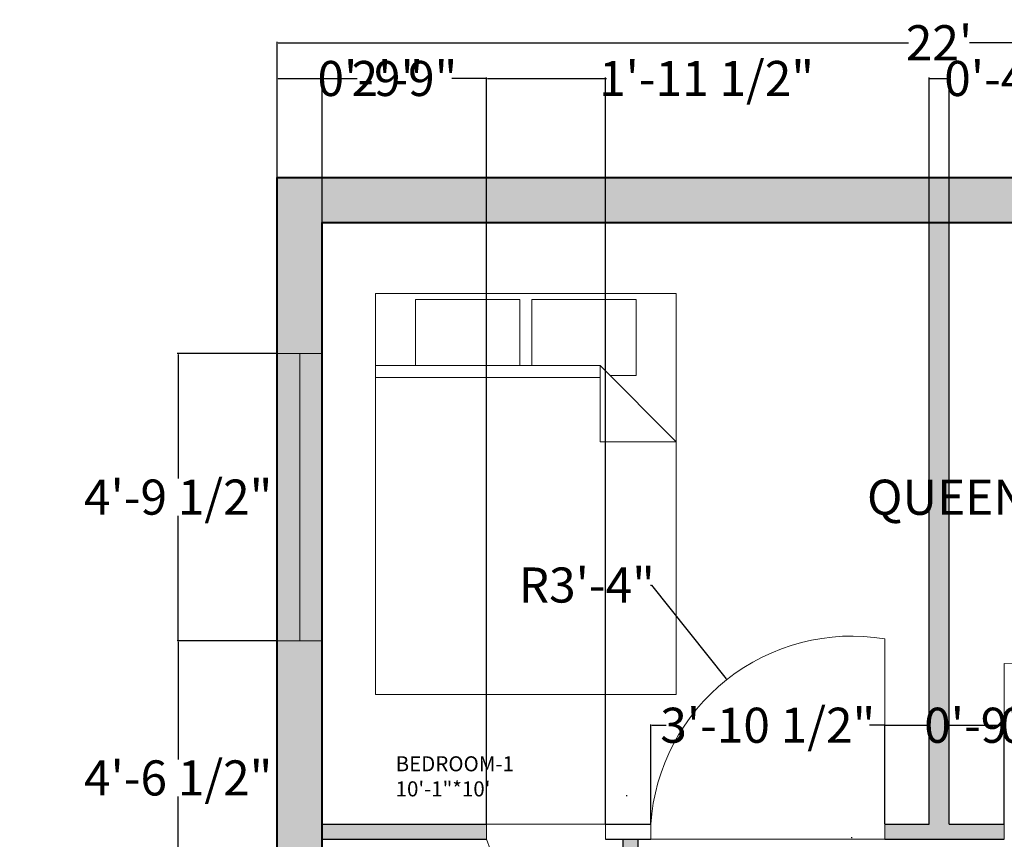
# Model space of a CAD drawing. Units: inches. Extents: x 4466 to 4826, y 3691 to 4152.
# Tile 3 of 4: x 4466 to 4663, y 3988 to 4152. Entities that reach past the tile are written whole.
import ezdxf

# ---------------------------------------------------------------- set-up
doc = ezdxf.new("R2010")
doc.units = ezdxf.units.IN
doc.header["$MEASUREMENT"] = 0
for name, color, linetype, lineweight in [('A-ANNO-DIMS', 2, 'Continuous', 13), ('A-DOOR', 3, 'Continuous', 18), ('A-FLOR-FIXT', 8, 'Continuous', 18), ('A-GLAZ', 4, 'Continuous', 13), ('A-GLAZ-PATT', 9, 'Continuous', 13), ('A-TEXT-ROOM', 7, 'Continuous', 18), ('A-WALL-EXTR', 7, 'Continuous', 40), ('A-WALL-INTR', 7, 'Continuous', 25), ('A-WALL-PATT', 251, 'Continuous', 13)]:
    doc.layers.add(name, color=color, linetype=linetype, lineweight=lineweight)
doc.styles.get("Standard").update_dxf_attribs({"font": 'arial.ttf'})
doc.dimstyles.get("Standard").update_dxf_attribs({"dimtxt": 7, "dimasz": 0.18, "dimexe": 0.18, "dimexo": 0.0625, "dimgap": 0.09, "dimtad": 0, "dimtih": 1, "dimtoh": 1, "dimdec": 0, "dimzin": 0, "dimdsep": 46, "dimlunit": 3, "dimtxsty": 'Standard', "dimcen": 0.09, "dimadec": 0, "dimazin": 0, "dimtfac": 1, "dimtdec": 0, "dimtofl": 0, "dimtmove": 0, "dimatfit": 3, "dimfxl": 1, "dimtolj": 1, "dimtzin": 0, "dimarcsym": 0})

# ---------------------------------------------------------------- blocks, each defined once
blk = doc.blocks.new('Bed - Queen')
for p, q in [((0, -80.00003), (0, 0)), ((0, 0), (59.99999, 0)), ((59.99999, 0), (59.99999, -80.00003)), ((7.99999, -1.2), (28.79998, -1.2)), ((7.99999, -14.4), (7.99999, -1.2)), ((28.79998, -1.2), (28.79998, -14.4)), ((31.19999, -1.2), (51.99999, -1.2)), ((31.19999, -14.4), (31.19999, -1.2)), ((51.99999, -1.2), (51.99999, -16.4)), ((0, -14.4), (44.8, -14.4)), ((59.99999, -29.6), (44.8, -14.4)), ((44.8, -14.4), (44.8, -29.6)), ((44.8, -16.8), (0, -16.8)), ((51.99999, -16.4), (46.79936, -16.4)), ((44.8, -29.6), (59.99999, -29.6)), ((59.99999, -80.00003), (0, -80.00003))]:
    blk.add_line(p, q)
blk = doc.blocks.new('*D7')
at = {"layer": 'A-ANNO-DIMS', "color": 0, "lineweight": -2, "transparency": 16777216}
for p, q in [((4517.73, 4120.34), (4517.73, 4147.34)), ((4517.91, 4147.16), (4643.64, 4147.16)), ((4781.55, 4147.16), (4655.82, 4147.16)), ((4781.73, 4120.34), (4781.73, 4147.34))]:
    blk.add_line(p, q, dxfattribs=at)
at = {"layer": 'A-ANNO-DIMS', "color": 0, "transparency": 16777216}
for points in [[(4517.91, 4147.19), (4517.91, 4147.13), (4517.73, 4147.16)], [(4781.55, 4147.19), (4781.55, 4147.13), (4781.73, 4147.16)]]:
    blk.add_solid(points, dxfattribs=at)
at = {"layer": 'Defpoints', "color": 0, "transparency": 16777216}
for p in [(4781.73, 4147.16), (4517.73, 4120.28), (4781.73, 4120.28)]:
    blk.add_point(p, dxfattribs=at)
at = {"layer": 'A-ANNO-DIMS', "color": 0, "transparency": 16777216, "insert": (4649.73, 4147.16), "char_height": 7, "attachment_point": 5}
blk.add_mtext("\\A1;22'", dxfattribs=at)
blk = doc.blocks.new('*D8')
at = {"layer": 'A-ANNO-DIMS', "color": 0, "lineweight": -2, "transparency": 16777216}
for p, q in [((4696.1, 4096.51), (4683.98, 4096.51)), ((4684.16, 4096.33), (4684.16, 4060.43)), ((4684.16, 4016.69), (4684.16, 4052.59)), ((4696.1, 4016.51), (4683.98, 4016.51))]:
    blk.add_line(p, q, dxfattribs=at)
at = {"layer": 'A-ANNO-DIMS', "color": 0, "transparency": 16777216}
for points in [[(4684.13, 4096.33), (4684.19, 4096.33), (4684.16, 4096.51)], [(4684.13, 4016.69), (4684.19, 4016.69), (4684.16, 4016.51)]]:
    blk.add_solid(points, dxfattribs=at)
at = {"layer": 'Defpoints', "color": 0, "transparency": 16777216}
for p in [(4684.16, 4096.51), (4696.16, 4096.51), (4696.16, 4016.51)]:
    blk.add_point(p, dxfattribs=at)
at = {"layer": 'A-ANNO-DIMS', "color": 0, "transparency": 16777216, "insert": (4684.16, 4056.51), "char_height": 7, "attachment_point": 5}
blk.add_mtext('\\A1;QUEEN BED 6\'-8" TYP.', dxfattribs=at)
blk = doc.blocks.new('*D10')
at = {"layer": 'A-ANNO-DIMS', "color": 0, "lineweight": -2, "transparency": 16777216}
for p, q in [((4527.05, 3975.44), (4526.87, 3975.44)), ((4527.05, 3970.54), (4527.05, 3975.62)), ((4559.92, 3975.44), (4527.23, 3975.44)), ((4560.1, 3970.54), (4560.1, 3975.62))]:
    blk.add_line(p, q, dxfattribs=at)
at = {"layer": 'A-ANNO-DIMS', "color": 0, "transparency": 16777216}
for points in [[(4527.23, 3975.47), (4527.23, 3975.41), (4527.05, 3975.44)], [(4559.92, 3975.47), (4559.92, 3975.41), (4560.1, 3975.44)]]:
    blk.add_solid(points, dxfattribs=at)
at = {"layer": 'Defpoints', "color": 0, "transparency": 16777216}
for p in [(4527.05, 3975.44), (4527.05, 3970.48), (4560.1, 3970.48)]:
    blk.add_point(p, dxfattribs=at)
at = {"layer": 'A-ANNO-DIMS', "color": 0, "transparency": 16777216, "insert": (4495.8, 3975.44), "char_height": 7, "attachment_point": 5}
blk.add_mtext('\\A1;WC 2\'-9" TYP.', dxfattribs=at)
blk = doc.blocks.new('*D26')
at = {"layer": 'A-ANNO-DIMS', "color": 0, "lineweight": -2, "transparency": 16777216}
for p, q in [((4517.67, 4027.88), (4497.8, 4027.88)), ((4497.98, 4027.7), (4497.98, 4004.23)), ((4497.98, 3973.33), (4497.98, 3996.81)), ((4517.67, 3973.15), (4497.8, 3973.15))]:
    blk.add_line(p, q, dxfattribs=at)
at = {"layer": 'A-ANNO-DIMS', "color": 0, "transparency": 16777216}
for points in [[(4497.95, 4027.7), (4498.01, 4027.7), (4497.98, 4027.88)], [(4497.95, 3973.33), (4498.01, 3973.33), (4497.98, 3973.15)]]:
    blk.add_solid(points, dxfattribs=at)
at = {"layer": 'Defpoints', "color": 0, "transparency": 16777216}
for p in [(4497.98, 4027.88), (4517.73, 4027.88), (4517.73, 3973.15)]:
    blk.add_point(p, dxfattribs=at)
at = {"layer": 'A-ANNO-DIMS', "color": 0, "transparency": 16777216, "insert": (4497.98, 4000.52), "char_height": 7, "attachment_point": 5}
blk.add_mtext('\\A1;4\'-6 1/2"', dxfattribs=at)
blk = doc.blocks.new('*D27')
at = {"layer": 'A-ANNO-DIMS', "color": 0, "lineweight": -2, "transparency": 16777216}
for p, q in [((4517.67, 4085.19), (4497.8, 4085.19)), ((4497.98, 4085.01), (4497.98, 4060.24)), ((4497.98, 4028.06), (4497.98, 4052.82)), ((4517.67, 4027.88), (4497.8, 4027.88))]:
    blk.add_line(p, q, dxfattribs=at)
at = {"layer": 'A-ANNO-DIMS', "color": 0, "transparency": 16777216}
for points in [[(4497.95, 4085.01), (4498.01, 4085.01), (4497.98, 4085.19)], [(4497.95, 4028.06), (4498.01, 4028.06), (4497.98, 4027.88)]]:
    blk.add_solid(points, dxfattribs=at)
at = {"layer": 'Defpoints', "color": 0, "transparency": 16777216}
for p in [(4497.98, 4085.19), (4517.73, 4085.19), (4517.73, 4027.88)]:
    blk.add_point(p, dxfattribs=at)
at = {"layer": 'A-ANNO-DIMS', "color": 0, "transparency": 16777216, "insert": (4497.98, 4056.53), "char_height": 7, "attachment_point": 5}
blk.add_mtext('\\A1;4\'-9 1/2"', dxfattribs=at)
blk = doc.blocks.new('*D44')
at = {"layer": 'A-ANNO-DIMS', "color": 0, "lineweight": -2, "transparency": 16777216}
for p, q in [((4559.49, 3991.34), (4559.49, 4140.21)), ((4559.67, 4140.03), (4583.06, 4140.03)), ((4583.24, 3991.34), (4583.24, 4140.21)), ((4583.24, 4140.03), (4583.42, 4140.03))]:
    blk.add_line(p, q, dxfattribs=at)
at = {"layer": 'A-ANNO-DIMS', "color": 0, "transparency": 16777216}
for points in [[(4559.67, 4140.06), (4559.67, 4140), (4559.49, 4140.03)], [(4583.06, 4140.06), (4583.06, 4140), (4583.24, 4140.03)]]:
    blk.add_solid(points, dxfattribs=at)
at = {"layer": 'Defpoints', "color": 0, "transparency": 16777216}
for p in [(4583.24, 4140.03), (4559.49, 3991.28), (4583.24, 3991.28)]:
    blk.add_point(p, dxfattribs=at)
at = {"layer": 'A-ANNO-DIMS', "color": 0, "transparency": 16777216, "insert": (4603.36, 4140.03), "char_height": 7, "attachment_point": 5}
blk.add_mtext('\\A1;1\'-11 1/2"', dxfattribs=at)
blk = doc.blocks.new('*D45')
at = {"layer": 'A-ANNO-DIMS', "color": 0, "lineweight": -2, "transparency": 16777216}
for p, q in [((4526.73, 3991.34), (4526.73, 4140.21)), ((4526.91, 4140.03), (4533.66, 4140.03)), ((4559.31, 4140.03), (4552.57, 4140.03)), ((4559.49, 3991.34), (4559.49, 4140.21))]:
    blk.add_line(p, q, dxfattribs=at)
at = {"layer": 'A-ANNO-DIMS', "color": 0, "transparency": 16777216}
for points in [[(4526.91, 4140.06), (4526.91, 4140), (4526.73, 4140.03)], [(4559.31, 4140.06), (4559.31, 4140), (4559.49, 4140.03)]]:
    blk.add_solid(points, dxfattribs=at)
at = {"layer": 'Defpoints', "color": 0, "transparency": 16777216}
for p in [(4559.49, 4140.03), (4526.73, 3991.28), (4559.49, 3991.28)]:
    blk.add_point(p, dxfattribs=at)
at = {"layer": 'A-ANNO-DIMS', "color": 0, "transparency": 16777216, "insert": (4543.11, 4140.03), "char_height": 7, "attachment_point": 5}
blk.add_mtext('\\A1;2\'-9"', dxfattribs=at)
blk = doc.blocks.new('*D47')
at = {"layer": 'A-ANNO-DIMS', "color": 0, "lineweight": -2, "transparency": 16777216}
for p, q in [((4517.73, 4120.34), (4517.73, 4140.21)), ((4517.91, 4140.03), (4526.55, 4140.03)), ((4526.73, 4111.34), (4526.73, 4140.21)), ((4526.73, 4140.03), (4526.91, 4140.03))]:
    blk.add_line(p, q, dxfattribs=at)
at = {"layer": 'A-ANNO-DIMS', "color": 0, "transparency": 16777216}
for points in [[(4517.91, 4140.06), (4517.91, 4140), (4517.73, 4140.03)], [(4526.55, 4140.06), (4526.55, 4140), (4526.73, 4140.03)]]:
    blk.add_solid(points, dxfattribs=at)
at = {"layer": 'Defpoints', "color": 0, "transparency": 16777216}
for p in [(4526.73, 4140.03), (4517.73, 4120.28), (4526.73, 4111.28)]:
    blk.add_point(p, dxfattribs=at)
at = {"layer": 'A-ANNO-DIMS', "color": 0, "transparency": 16777216, "insert": (4536.31, 4140.03), "char_height": 7, "attachment_point": 5}
blk.add_mtext('\\A1;0\'-9"', dxfattribs=at)
blk = doc.blocks.new('*D48')
at = {"layer": 'A-ANNO-DIMS', "color": 0, "lineweight": -2, "transparency": 16777216}
for p, q in [((4647.73, 4111.34), (4647.73, 4140.21)), ((4647.91, 4140.03), (4651.55, 4140.03)), ((4651.73, 4111.34), (4651.73, 4140.21)), ((4651.73, 4140.03), (4651.91, 4140.03))]:
    blk.add_line(p, q, dxfattribs=at)
at = {"layer": 'A-ANNO-DIMS', "color": 0, "transparency": 16777216}
for points in [[(4647.91, 4140.06), (4647.91, 4140), (4647.73, 4140.03)], [(4651.55, 4140.06), (4651.55, 4140), (4651.73, 4140.03)]]:
    blk.add_solid(points, dxfattribs=at)
at = {"layer": 'Defpoints', "color": 0, "transparency": 16777216}
for p in [(4651.73, 4140.03), (4647.73, 4111.28), (4651.73, 4111.28)]:
    blk.add_point(p, dxfattribs=at)
at = {"layer": 'A-ANNO-DIMS', "color": 0, "transparency": 16777216, "insert": (4661.31, 4140.03), "char_height": 7, "attachment_point": 5}
blk.add_mtext('\\A1;0\'-4"', dxfattribs=at)
blk = doc.blocks.new('*D49')
at = {"layer": 'A-ANNO-DIMS', "color": 0, "lineweight": -2, "transparency": 16777216}
for p, q in [((4592.25, 3991.34), (4592.25, 4011.21)), ((4592.43, 4011.03), (4595.31, 4011.03)), ((4638.72, 4011.03), (4635.84, 4011.03)), ((4638.9, 3991.34), (4638.9, 4011.21))]:
    blk.add_line(p, q, dxfattribs=at)
at = {"layer": 'A-ANNO-DIMS', "color": 0, "transparency": 16777216}
for points in [[(4592.43, 4011.06), (4592.43, 4011), (4592.25, 4011.03)], [(4638.72, 4011.06), (4638.72, 4011), (4638.9, 4011.03)]]:
    blk.add_solid(points, dxfattribs=at)
at = {"layer": 'Defpoints', "color": 0, "transparency": 16777216}
for p in [(4638.9, 4011.03), (4592.25, 3991.28), (4638.9, 3991.28)]:
    blk.add_point(p, dxfattribs=at)
at = {"layer": 'A-ANNO-DIMS', "color": 0, "transparency": 16777216, "insert": (4615.57, 4011.03), "char_height": 7, "attachment_point": 5}
blk.add_mtext('\\A1;3\'-10 1/2"', dxfattribs=at)
blk = doc.blocks.new('*D50')
at = {"layer": 'A-ANNO-DIMS', "color": 0, "lineweight": -2, "transparency": 16777216}
for p, q in [((4638.9, 3991.34), (4638.9, 4011.21)), ((4639.08, 4011.03), (4647.55, 4011.03)), ((4647.73, 3991.34), (4647.73, 4011.21)), ((4647.73, 4011.03), (4647.91, 4011.03))]:
    blk.add_line(p, q, dxfattribs=at)
at = {"layer": 'A-ANNO-DIMS', "color": 0, "transparency": 16777216}
for points in [[(4639.08, 4011.06), (4639.08, 4011), (4638.9, 4011.03)], [(4647.55, 4011.06), (4647.55, 4011), (4647.73, 4011.03)]]:
    blk.add_solid(points, dxfattribs=at)
at = {"layer": 'Defpoints', "color": 0, "transparency": 16777216}
for p in [(4647.73, 4011.03), (4638.9, 3991.28), (4647.73, 3991.28)]:
    blk.add_point(p, dxfattribs=at)
at = {"layer": 'A-ANNO-DIMS', "color": 0, "transparency": 16777216, "insert": (4657.31, 4011.03), "char_height": 7, "attachment_point": 5}
blk.add_mtext('\\A1;0\'-9"', dxfattribs=at)
blk = doc.blocks.new('*D51')
at = {"layer": 'A-ANNO-DIMS', "color": 0, "lineweight": -2, "transparency": 16777216}
for p, q in [((4651.73, 3991.34), (4651.73, 4011.21)), ((4651.91, 4011.03), (4662.57, 4011.03)), ((4662.75, 3991.34), (4662.75, 4011.21)), ((4662.75, 4011.03), (4662.93, 4011.03))]:
    blk.add_line(p, q, dxfattribs=at)
at = {"layer": 'A-ANNO-DIMS', "color": 0, "transparency": 16777216}
for points in [[(4651.91, 4011.06), (4651.91, 4011), (4651.73, 4011.03)], [(4662.57, 4011.06), (4662.57, 4011), (4662.75, 4011.03)]]:
    blk.add_solid(points, dxfattribs=at)
at = {"layer": 'Defpoints', "color": 0, "transparency": 16777216}
for p in [(4662.75, 4011.03), (4651.73, 3991.28), (4662.75, 3991.28)]:
    blk.add_point(p, dxfattribs=at)
at = {"layer": 'A-ANNO-DIMS', "color": 0, "transparency": 16777216, "insert": (4675.04, 4011.03), "char_height": 7, "attachment_point": 5}
blk.add_mtext('\\A1;0\'-11"', dxfattribs=at)
blk = doc.blocks.new('*D62')
at = {"layer": 'A-ANNO-DIMS', "color": 0, "lineweight": -2, "transparency": 16777216}
for p, q in [((4592.21, 4039), (4592.39, 4039)), ((4592.39, 4039), (4607.26, 4020.26)), ((4632.24, 3988.64), (4632.42, 3988.64)), ((4632.33, 3988.55), (4632.33, 3988.73))]:
    blk.add_line(p, q, dxfattribs=at)
at = {"layer": 'A-ANNO-DIMS', "color": 0, "transparency": 16777216}
blk.add_solid([(4607.28, 4020.28), (4607.24, 4020.24), (4607.37, 4020.12)], dxfattribs=at)
at = {"layer": 'Defpoints', "color": 0, "transparency": 16777216}
for p in [(4607.37, 4020.12), (4632.33, 3988.64)]:
    blk.add_point(p, dxfattribs=at)
at = {"layer": 'A-ANNO-DIMS', "color": 0, "transparency": 16777216, "insert": (4579.47, 4039), "char_height": 7, "attachment_point": 5}
blk.add_mtext('\\A1;R3\'-4"', dxfattribs=at)
blk = doc.blocks.new('*D63')
at = {"layer": 'A-ANNO-DIMS', "color": 0, "lineweight": -2, "transparency": 16777216}
for p, q in [((4587.35, 3996.99), (4587.53, 3996.99)), ((4587.44, 3996.9), (4587.44, 3997.08)), ((4557.04, 3961.36), (4568.32, 3974.59)), ((4556.86, 3961.36), (4557.04, 3961.36))]:
    blk.add_line(p, q, dxfattribs=at)
at = {"layer": 'A-ANNO-DIMS', "color": 0, "transparency": 16777216}
blk.add_solid([(4568.3, 3974.6), (4568.35, 3974.57), (4568.44, 3974.72)], dxfattribs=at)
at = {"layer": 'Defpoints', "color": 0, "transparency": 16777216}
for p in [(4587.44, 3996.99), (4568.44, 3974.72)]:
    blk.add_point(p, dxfattribs=at)
at = {"layer": 'A-ANNO-DIMS', "color": 0, "transparency": 16777216, "insert": (4535.96, 3961.36), "char_height": 7, "attachment_point": 5}
blk.add_mtext('\\A1;R2\'-5 1/2"', dxfattribs=at)

msp = doc.modelspace()

# ---------------------------------------------------------------- hatches: boundary and pattern name
at = {"layer": 'A-GLAZ-PATT'}
h = msp.add_hatch(color=256, dxfattribs=at)
h.dxf.hatch_style = 1
h.paths.add_polyline_path([(4781.73, 3815.6), (4777.23, 3815.6), (4777.23, 3780.77), (4781.73, 3780.77)])
h.paths.add_polyline_path([(4777.23, 3815.6), (4772.73, 3815.6), (4772.73, 3780.77), (4777.23, 3780.77)])
h.paths.add_polyline_path([(4781.73, 3906.43), (4777.23, 3906.43), (4777.23, 3867), (4781.73, 3867)])
h.paths.add_polyline_path([(4777.23, 3906.43), (4772.73, 3906.43), (4772.73, 3867), (4777.23, 3867)])
h.paths.add_polyline_path([(4777.23, 3975.56), (4772.73, 3975.56), (4772.73, 3940.28), (4777.23, 3940.28)])
h.paths.add_polyline_path([(4781.73, 3975.56), (4777.23, 3975.56), (4777.23, 3940.28), (4781.73, 3940.28)])
h.paths.add_polyline_path([(4781.73, 4086.44), (4777.23, 4086.44), (4777.23, 4025.83), (4781.73, 4025.83)])
h.paths.add_polyline_path([(4777.23, 4086.44), (4772.73, 4086.44), (4772.73, 4025.83), (4777.23, 4025.83)])
h.paths.add_polyline_path([(4526.73, 4085.19), (4522.23, 4085.19), (4522.23, 4027.88), (4526.73, 4027.88)])
h.paths.add_polyline_path([(4522.23, 4085.19), (4517.73, 4085.19), (4517.73, 4027.88), (4522.23, 4027.88)])
h.paths.add_polyline_path([(4526.73, 3973.15), (4522.23, 3973.15), (4522.23, 3949.75), (4526.73, 3949.75)])
h.paths.add_polyline_path([(4522.23, 3973.15), (4517.73, 3973.15), (4517.73, 3949.75), (4522.23, 3949.75)])
h.paths.add_polyline_path([(4522.23, 3906.82), (4517.73, 3906.82), (4517.73, 3871.98), (4522.23, 3871.98)])
h.paths.add_polyline_path([(4526.73, 3906.82), (4522.23, 3906.82), (4522.23, 3871.98), (4526.73, 3871.98)])
h.paths.add_polyline_path([(4526.73, 3829.25), (4522.23, 3829.25), (4522.23, 3789.34), (4526.73, 3789.34)])
h.paths.add_polyline_path([(4522.23, 3829.25), (4517.73, 3829.25), (4517.73, 3789.34), (4522.23, 3789.34)])
at = {"layer": 'A-WALL-PATT'}
h = msp.add_hatch(color=256, dxfattribs=at)
h.dxf.hatch_style = 1
h.paths.add_polyline_path([(4781.73, 4120.28), (4517.73, 4120.28), (4517.73, 4085.19), (4526.73, 4085.19), (4526.73, 4111.28), (4772.73, 4111.28), (4772.73, 4086.44), (4781.73, 4086.44)])
h.paths.add_polyline_path([(4526.73, 4027.88), (4517.73, 4027.88), (4517.73, 3973.15), (4526.73, 3973.15)])
h.paths.add_polyline_path([(4781.73, 4025.83), (4772.73, 4025.83), (4772.73, 3975.56), (4781.73, 3975.56)])
h.paths.add_polyline_path([(4651.73, 4111.28), (4647.73, 4111.28), (4647.73, 3991.28), (4638.9, 3991.28), (4638.9, 3988.28), (4662.75, 3988.28), (4662.75, 3991.28), (4651.73, 3991.28)])
h.paths.add_polyline_path([(4781.73, 3780.77), (4772.73, 3780.77), (4772.73, 3769.28), (4657.39, 3769.28), (4657.39, 3760.28), (4781.73, 3760.28)])
h.paths.add_polyline_path([(4781.73, 3867), (4772.73, 3867), (4772.73, 3815.6), (4781.73, 3815.6)])
h.paths.add_polyline_path([(4781.73, 3940.28), (4772.73, 3940.28), (4772.73, 3906.43), (4781.73, 3906.43)])
h.paths.add_polyline_path([(4526.73, 3949.75), (4517.73, 3949.75), (4517.73, 3906.82), (4526.73, 3906.82)])
h.paths.add_polyline_path([(4526.73, 3871.98), (4517.73, 3871.98), (4517.73, 3829.25), (4526.73, 3829.25)])
h.paths.add_polyline_path([(4618.18, 3769.28), (4526.73, 3769.28), (4526.73, 3789.34), (4517.73, 3789.34), (4517.73, 3760.28), (4618.18, 3760.28)])
h.paths.add_polyline_path([(4576.17, 3850.28), (4526.73, 3850.28), (4526.73, 3847.28), (4576.17, 3847.28)])
h.paths.add_polyline_path([(4613.73, 3825.64), (4618.18, 3825.64), (4618.18, 3828.64), (4613.73, 3828.64), (4613.73, 3850.28), (4610.73, 3850.28), (4606.34, 3850.28), (4606.34, 3847.28), (4610.73, 3847.28), (4610.73, 3769.28), (4613.73, 3769.28)])
h.paths.add_polyline_path([(4772.73, 3828.64), (4657.39, 3828.64), (4657.39, 3825.64), (4772.73, 3825.64)])
h.paths.add_polyline_path([(4589.73, 3988.28), (4586.73, 3988.28), (4586.73, 3928.28), (4589.73, 3928.28)])
h.paths.add_polyline_path([(4712.73, 3956.78), (4709.73, 3956.78), (4709.73, 3925.28), (4772.73, 3925.28), (4772.73, 3928.28), (4712.73, 3928.28)])
h.paths.add_polyline_path([(4772.73, 3991.28), (4705.82, 3991.28), (4705.82, 3988.28), (4772.73, 3988.28)])
h.paths.add_polyline_path([(4559.49, 3991.28), (4526.73, 3991.28), (4526.73, 3988.28), (4559.49, 3988.28)])

# ---------------------------------------------------------------- linework, layer by layer
at = {"layer": 'A-DOOR'}
for p, q in [((4638.9, 4015.64), (4638.9, 4028.28)), ((4662.75, 3991.28), (4662.75, 4023.34)), ((4638.9, 3991.28), (4638.9, 4015.64)), ((4559.49, 3991.28), (4559.49, 3988.28)), ((4559.49, 3991.28), (4583.24, 3991.28)), ((4583.24, 3988.28), (4583.24, 3991.28)), ((4592.25, 3988.28), (4592.25, 3991.28)), ((4638.9, 3991.28), (4638.9, 3988.28)), ((4662.75, 3991.28), (4662.75, 3988.28)), ((4592.25, 3988.28), (4638.9, 3988.28))]:
    msp.add_line(p, q, dxfattribs=at)
for centre, radius, start, end in [((4632.33, 3988.64), 40.17, 80.5995, 176.2392), ((4663.3, 3979.11), 44.22, 15.9662, 90.7121), ((4587.44, 3996.99), 29.27, 197.3221, 261.7576)]:
    msp.add_arc(centre, radius, start, end, dxfattribs=at)
at = {"layer": 'A-GLAZ'}
for p, q in [((4517.73, 4085.19), (4526.73, 4085.19)), ((4522.23, 4085.19), (4522.23, 4027.88)), ((4517.73, 4027.88), (4526.73, 4027.88))]:
    msp.add_line(p, q, dxfattribs=at)
at = {"layer": 'A-WALL-EXTR'}
for p, q in [((4526.73, 4111.28), (4772.73, 4111.28)), ((4526.73, 3769.28), (4526.73, 4111.28))]:
    msp.add_line(p, q, dxfattribs=at)
msp.add_lwpolyline([(4618.18, 3760.28), (4517.73, 3760.28), (4517.73, 4120.28), (4781.73, 4120.28), (4781.73, 3760.28), (4657.39, 3760.28)], dxfattribs=at)
at = {"layer": 'A-WALL-INTR'}
for p, q in [((4647.73, 3991.28), (4647.73, 4111.28)), ((4651.73, 3991.28), (4651.73, 4111.28)), ((4526.73, 3991.28), (4559.49, 3991.28)), ((4583.24, 3991.28), (4592.25, 3991.28)), ((4638.9, 3991.28), (4647.73, 3991.28)), ((4651.73, 3991.28), (4662.75, 3991.28)), ((4526.73, 3988.28), (4559.49, 3988.28)), ((4583.24, 3988.28), (4592.25, 3988.28)), ((4586.73, 3928.28), (4586.73, 3988.28)), ((4589.73, 3928.28), (4589.73, 3988.28)), ((4638.9, 3988.28), (4662.75, 3988.28))]:
    msp.add_line(p, q, dxfattribs=at)

# ---------------------------------------------------------------- block references
at = {"layer": 'A-FLOR-FIXT'}
msp.add_blockref('Bed - Queen', (4537.33, 4097.16), dxfattribs=at)

# ---------------------------------------------------------------- texts
at = {"layer": 'A-TEXT-ROOM', "insert": (4541.35, 4004.84), "char_height": 3, "attachment_point": 1}
msp.add_mtext_dynamic_manual_height_columns('BEDROOM-1\\P10\'-1"*10\'', width=77.4792, gutter_width=1, heights=[0], dxfattribs=at)

# ---------------------------------------------------------------- dimensions: what is measured, and where the dimension line sits
at = {"layer": 'A-ANNO-DIMS'}
for base, p1, p2, override, picture, middle in [((4781.73, 4147.16), (4517.73, 4120.28), (4781.73, 4120.28), {"dimclrd": 0, "dimclre": 0, "dimclrt": 0}, '*D7', (4649.73, 4147.16)), ((4583.24, 4140.0291), (4559.4911, 3991.2791), (4583.24, 3991.2791), {"dimdec": 1, "dimlfac": 1, "dimrnd": 0, "dimzin": 1, "dimdsep": 46, "dimlunit": 4, "dimfrac": 2}, '*D44', (4603.3592, 4140.0291)), ((4526.73, 4140.03), (4517.73, 4120.28), (4526.73, 4111.28), {"dimdec": 1, "dimlfac": 1, "dimrnd": 0, "dimzin": 1, "dimdsep": 46, "dimlunit": 4, "dimfrac": 2}, '*D47', (4536.31, 4140.03)), ((4559.49, 4140.03), (4526.73, 3991.28), (4559.49, 3991.28), {"dimdec": 1, "dimlfac": 1, "dimrnd": 0, "dimzin": 1, "dimdsep": 46, "dimlunit": 4, "dimfrac": 2}, '*D45', (4543.11, 4140.03)), ((4651.73, 4140.03), (4647.73, 4111.28), (4651.73, 4111.28), {"dimdec": 1, "dimlfac": 1, "dimrnd": 0, "dimzin": 1, "dimdsep": 46, "dimlunit": 4, "dimfrac": 2}, '*D48', (4661.31, 4140.03)), ((4638.8964, 4011.0291), (4592.2485, 3991.2791), (4638.8964, 3991.2791), {"dimdec": 1, "dimlfac": 1, "dimrnd": 0, "dimzin": 1, "dimdsep": 46, "dimlunit": 4, "dimfrac": 2}, '*D49', (4615.5724, 4011.0291)), ((4647.73, 4011.03), (4638.9, 3991.28), (4647.73, 3991.28), {"dimdec": 1, "dimlfac": 1, "dimrnd": 0, "dimzin": 1, "dimdsep": 46, "dimlunit": 4, "dimfrac": 2}, '*D50', (4657.31, 4011.03))]:
    dim = msp.add_linear_dim(base=base, p1=p1, p2=p2, dimstyle='Standard', override=override, dxfattribs=at)
    dim.commit()
    dim.dimension.update_dxf_attribs({"geometry": picture, "text_midpoint": middle})
for base, p1, p2, angle, text, picture, middle in [((4684.16, 4096.51), (4696.16, 4016.51), (4696.16, 4096.51), 90, 'QUEEN BED <> TYP.', '*D8', (4684.16, 4056.51)), ((4527.0496, 3975.4363), (4560.0959, 3970.4794), (4527.0496, 3970.4794), 180, 'WC <> TYP.', '*D10', (4495.7977, 3975.4363))]:
    dim = msp.add_linear_dim(base=base, p1=p1, p2=p2, angle=angle, text=text, dimstyle='Standard', override={"dimdec": 1, "dimlfac": 1, "dimrnd": 0, "dimzin": 1, "dimdsep": 46, "dimlunit": 4, "dimfrac": 2}, dxfattribs=at)
    dim.commit()
    dim.dimension.update_dxf_attribs({"geometry": picture, "text_midpoint": middle})
for base, p1, p2, angle, picture, middle in [((4497.98, 4085.19), (4517.73, 4027.88), (4517.73, 4085.19), 90, '*D27', (4497.98, 4056.53)), ((4497.98, 4027.88), (4517.73, 3973.15), (4517.73, 4027.88), 90, '*D26', (4497.98, 4000.52)), ((4662.75, 4011.03), (4651.73, 3991.28), (4662.75, 3991.28), 0, '*D51', (4675.04, 4011.03))]:
    dim = msp.add_linear_dim(base=base, p1=p1, p2=p2, angle=angle, dimstyle='Standard', override={"dimdec": 1, "dimlfac": 1, "dimrnd": 0, "dimzin": 1, "dimdsep": 46, "dimlunit": 4, "dimfrac": 2}, dxfattribs=at)
    dim.commit()
    dim.dimension.update_dxf_attribs({"geometry": picture, "text_midpoint": middle})
for center, mpoint, picture, middle in [((4632.33, 3988.64), (4607.37, 4020.12), '*D62', (4579.47, 4039)), ((4587.44, 3996.99), (4568.44, 3974.72), '*D63', (4535.96, 3961.36))]:
    dim = msp.add_radius_dim(center=center, mpoint=mpoint, dimstyle='Standard', override={"dimdec": 1, "dimlfac": 1, "dimrnd": 0, "dimzin": 1, "dimdsep": 46, "dimlunit": 4, "dimfrac": 2}, dxfattribs=at)
    dim.commit()
    dim.dimension.update_dxf_attribs({"geometry": picture, "text_midpoint": middle, "dimtype": 164})

doc.saveas('drawing.dxf')
